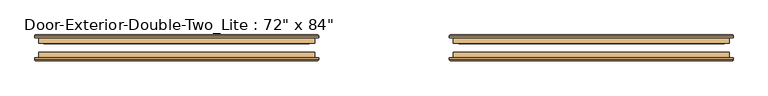
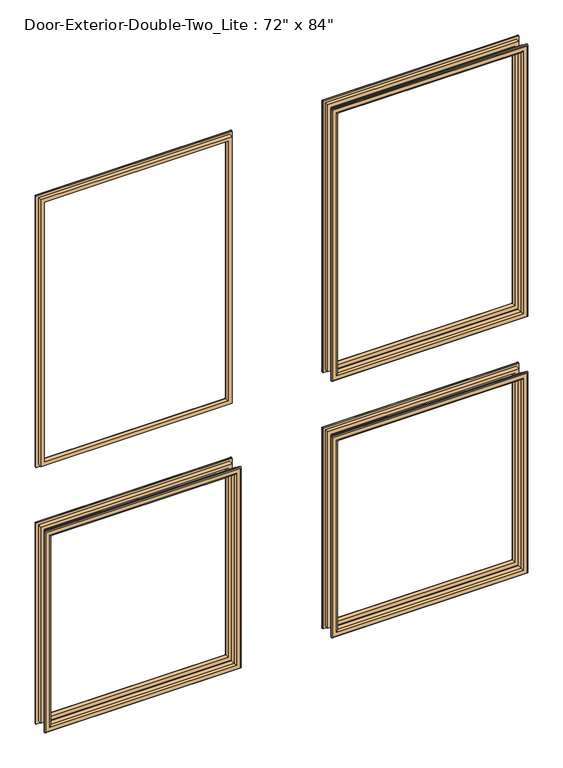
"""IFC4 building model written with IfcOpenShell, lengths in millimetres: door geometry."""

from ifc_helpers import new_model, si_unit, frame, origin, place, context, project, spatial, ellipse_curve, source, transform, mapped, element, save
from ifc_brep_helpers import plane_surface, cylinder_surface, advanced_brep


def door_549a8064(model_context):
    return source(origin(), model_context, "Body", "AdvancedBrep", [
        advanced_brep(
        [(-762.0, 69.85, 914.4), (-762.0, 82.55, 914.4), (-762.0, 82.55, 254.0), (-762.0, 69.85, 254.0), (-750.0, 83.55, 902.4), (-750.0, 69.85, 902.4), (-750.0, 69.85, 266.0), (-750.0, 83.55, 266.0), (-755.0, 88.55, 907.4), (-755.0, 88.55, 261.0), (-770.0, 86.55, 922.4), (-768.0, 88.55, 920.4), (-768.0, 88.55, 248.0), (-770.0, 86.55, 246.0), (-770.0, 82.55, 922.4), (-770.0, 82.55, 246.0), (-152.4, 82.55, 254.0), (-152.4, 69.85, 254.0), (-164.4, 69.85, 266.0), (-164.4, 83.55, 266.0), (-159.4, 88.55, 261.0), (-146.4, 88.55, 248.0), (-144.4, 86.55, 246.0), (-144.4, 82.55, 246.0), (-152.4, 82.55, 914.4), (-152.4, 69.85, 914.4), (-164.4, 69.85, 902.4), (-164.4, 83.55, 902.4), (-159.4, 88.55, 907.4), (-146.4, 88.55, 920.4), (-144.4, 86.55, 922.4), (-144.4, 82.55, 922.4)],
        [
            (0, 1),
            (1, 2),
            (2, 3),
            (3, 0),
            (4, 5),
            (5, 6),
            (6, 7),
            (7, 4),
            (8, 4, ellipse_curve(frame((-755.0, 83.55, 907.4), z_axis=(-0.7071067811865475, 0.0, -0.7071067811865475), x_axis=(-0.7071067811865474, 0.0, 0.7071067811865476)), 7.0710678, 5.0)),
            (7, 9, ellipse_curve(frame((-755.0, 83.55, 261.0), z_axis=(-0.7071067811865475, 0.0, 0.7071067811865475), x_axis=(0.7071067811865474, 0.0, 0.7071067811865476)), 7.0710678, 5.0)),
            (9, 8),
            (10, 11, ellipse_curve(frame((-768.0, 86.55, 920.4), z_axis=(-0.7071067811865475, 0.0, -0.7071067811865475), x_axis=(-0.7071067811865474, 0.0, 0.7071067811865476)), 2.8284271, 2.0)),
            (11, 12),
            (12, 13, ellipse_curve(frame((-768.0, 86.55, 248.0), z_axis=(-0.7071067811865475, 0.0, 0.7071067811865475), x_axis=(0.7071067811865474, 0.0, 0.7071067811865476)), 2.8284271, 2.0)),
            (13, 10),
            (14, 10),
            (13, 15),
            (15, 14),
            (2, 16),
            (16, 17),
            (17, 3),
            (6, 18),
            (18, 19),
            (19, 7),
            (19, 20, ellipse_curve(frame((-159.4, 83.55, 261.0), z_axis=(-0.7071067811865475, 0.0, -0.7071067811865475), x_axis=(-0.7071067811865476, 0.0, 0.7071067811865474)), 7.0710678, 5.0)),
            (20, 9),
            (12, 21),
            (21, 22, ellipse_curve(frame((-146.4, 86.55, 248.0), z_axis=(-0.7071067811865475, 0.0, -0.7071067811865475), x_axis=(-0.7071067811865476, 0.0, 0.7071067811865474)), 2.8284271, 2.0)),
            (22, 13),
            (22, 23),
            (23, 15),
            (16, 24),
            (24, 25),
            (25, 17),
            (18, 26),
            (26, 27),
            (27, 19),
            (27, 28, ellipse_curve(frame((-159.4, 83.55, 907.4), z_axis=(0.7071067811865475, 0.0, -0.7071067811865475), x_axis=(-0.7071067811865474, 0.0, -0.7071067811865476)), 7.0710678, 5.0)),
            (28, 20),
            (21, 29),
            (29, 30, ellipse_curve(frame((-146.4, 86.55, 920.4), z_axis=(0.7071067811865475, 0.0, -0.7071067811865475), x_axis=(-0.7071067811865474, 0.0, -0.7071067811865476)), 2.8284271, 2.0)),
            (30, 22),
            (30, 31),
            (31, 23),
            (31, 14),
            (1, 24),
            (0, 25),
            (5, 26),
            (4, 27),
            (8, 28),
            (11, 29),
            (10, 30),
        ],
        [
            plane_surface(frame((-762.0, 82.55, 914.4), z_axis=(-1.0, 0.0, 0.0), x_axis=(0.0, 0.0, -1.0))),
            plane_surface(frame((-750.0, 69.85, 902.4), z_axis=(1.0, 0.0, 0.0), x_axis=(0.0, 0.0, -1.0))),
            cylinder_surface(frame((-755.0, 83.55, 914.4), z_axis=(0.0, 0.0, 1.0), x_axis=(-1.0, 0.0, 0.0)), 5.0),
            cylinder_surface(frame((-768.0, 86.55, 914.4), z_axis=(0.0, 0.0, 1.0), x_axis=(-1.0, 0.0, 0.0)), 2.0),
            plane_surface(frame((-770.0, 86.55, 922.4), z_axis=(-1.0, 0.0, 0.0), x_axis=(0.0, 0.0, -1.0))),
            plane_surface(frame((-762.0, 82.55, 254.0), z_axis=(0.0, 0.0, -1.0), x_axis=(1.0, 0.0, 0.0))),
            plane_surface(frame((-750.0, 69.85, 266.0), z_axis=(0.0, 0.0, 1.0), x_axis=(1.0, 0.0, 0.0))),
            cylinder_surface(frame((-762.0, 83.55, 261.0), z_axis=(-1.0, 0.0, 0.0), x_axis=(0.0, 0.0, -1.0)), 5.0),
            cylinder_surface(frame((-762.0, 86.55, 248.0), z_axis=(-1.0, 0.0, 0.0), x_axis=(0.0, 0.0, -1.0)), 2.0),
            plane_surface(frame((-770.0, 86.55, 246.0), z_axis=(0.0, 0.0, -1.0), x_axis=(1.0, 0.0, 0.0))),
            plane_surface(frame((-152.4, 82.55, 254.0), z_axis=(1.0, 0.0, 0.0), x_axis=(0.0, 0.0, 1.0))),
            plane_surface(frame((-164.4, 69.85, 266.0), z_axis=(-1.0, 0.0, 0.0), x_axis=(0.0, 0.0, 1.0))),
            cylinder_surface(frame((-159.4, 83.55, 254.0), z_axis=(0.0, 0.0, -1.0), x_axis=(1.0, 0.0, 0.0)), 5.0),
            cylinder_surface(frame((-146.4, 86.55, 254.0), z_axis=(0.0, 0.0, -1.0), x_axis=(1.0, 0.0, 0.0)), 2.0),
            plane_surface(frame((-144.4, 86.55, 246.0), z_axis=(1.0, 0.0, 0.0), x_axis=(0.0, 0.0, 1.0))),
            plane_surface(frame((-144.4, 82.55, 922.4), z_axis=(0.0, -1.0, 0.0), x_axis=(-1.0, 0.0, 0.0))),
            plane_surface(frame((-152.4, 82.55, 914.4), z_axis=(0.0, 0.0, 1.0), x_axis=(-1.0, 0.0, 0.0))),
            plane_surface(frame((-152.4, 69.85, 914.4), z_axis=(0.0, -1.0, 0.0), x_axis=(-1.0, 0.0, 0.0))),
            plane_surface(frame((-164.4, 69.85, 902.4), z_axis=(0.0, 0.0, -1.0), x_axis=(-1.0, 0.0, 0.0))),
            cylinder_surface(frame((-152.4, 83.55, 907.4), z_axis=(1.0, 0.0, 0.0), x_axis=(0.0, 0.0, 1.0)), 5.0),
            plane_surface(frame((-159.4, 88.55, 907.4), z_axis=(0.0, 1.0, 0.0), x_axis=(-1.0, 0.0, 0.0))),
            cylinder_surface(frame((-152.4, 86.55, 920.4), z_axis=(1.0, 0.0, 0.0), x_axis=(0.0, 0.0, 1.0)), 2.0),
            plane_surface(frame((-144.4, 86.55, 922.4), z_axis=(0.0, 0.0, 1.0), x_axis=(-1.0, 0.0, 0.0))),
        ],
        [
            (0, [[1, 2, 3, 4]]),
            (1, [[5, 6, 7, 8]]),
            (2, [[9, -8, 10, 11]]),
            (3, [[12, 13, 14, 15]]),
            (4, [[16, -15, 17, 18]]),
            (5, [[-3, 19, 20, 21]]),
            (6, [[-7, 22, 23, 24]]),
            (7, [[-10, -24, 25, 26]]),
            (8, [[-14, 27, 28, 29]]),
            (9, [[-17, -29, 30, 31]]),
            (10, [[-20, 32, 33, 34]]),
            (11, [[-23, 35, 36, 37]]),
            (12, [[-25, -37, 38, 39]]),
            (13, [[-28, 40, 41, 42]]),
            (14, [[-30, -42, 43, 44]]),
            (15, [[-31, -44, 45, -18], [46, -32, -19, -2]]),
            (16, [[-33, -46, -1, 47]]),
            (17, [[-21, -34, -47, -4], [48, -35, -22, -6]]),
            (18, [[-36, -48, -5, 49]]),
            (19, [[-38, -49, -9, 50]]),
            (20, [[51, -40, -27, -13], [-26, -39, -50, -11]]),
            (21, [[-41, -51, -12, 52]]),
            (22, [[-43, -52, -16, -45]]),
        ],
    ),
        advanced_brep(
        [(152.4, 69.85, 914.4), (152.4, 82.55, 914.4), (152.4, 82.55, 254.0), (152.4, 69.85, 254.0), (164.4, 83.55, 902.4), (164.4, 69.85, 902.4), (164.4, 69.85, 266.0), (164.4, 83.55, 266.0), (159.4, 88.55, 907.4), (159.4, 88.55, 261.0), (144.4, 86.55, 922.4), (146.4, 88.55, 920.4), (146.4, 88.55, 248.0), (144.4, 86.55, 246.0), (144.4, 82.55, 922.4), (144.4, 82.55, 246.0), (762.0, 82.55, 254.0), (762.0, 69.85, 254.0), (750.0, 69.85, 266.0), (750.0, 83.55, 266.0), (755.0, 88.55, 261.0), (768.0, 88.55, 248.0), (770.0, 86.55, 246.0), (770.0, 82.55, 246.0), (762.0, 82.55, 914.4), (762.0, 69.85, 914.4), (750.0, 69.85, 902.4), (750.0, 83.55, 902.4), (755.0, 88.55, 907.4), (768.0, 88.55, 920.4), (770.0, 86.55, 922.4), (770.0, 82.55, 922.4)],
        [
            (0, 1),
            (1, 2),
            (2, 3),
            (3, 0),
            (4, 5),
            (5, 6),
            (6, 7),
            (7, 4),
            (8, 4, ellipse_curve(frame((159.4, 83.55, 907.4), z_axis=(-0.7071067811865475, 0.0, -0.7071067811865475), x_axis=(-0.7071067811865474, 0.0, 0.7071067811865476)), 7.0710678, 5.0)),
            (7, 9, ellipse_curve(frame((159.4, 83.55, 261.0), z_axis=(-0.7071067811865475, 0.0, 0.7071067811865475), x_axis=(0.7071067811865474, 0.0, 0.7071067811865476)), 7.0710678, 5.0)),
            (9, 8),
            (10, 11, ellipse_curve(frame((146.4, 86.55, 920.4), z_axis=(-0.7071067811865475, 0.0, -0.7071067811865475), x_axis=(-0.7071067811865474, 0.0, 0.7071067811865476)), 2.8284271, 2.0)),
            (11, 12),
            (12, 13, ellipse_curve(frame((146.4, 86.55, 248.0), z_axis=(-0.7071067811865475, 0.0, 0.7071067811865475), x_axis=(0.7071067811865474, 0.0, 0.7071067811865476)), 2.8284271, 2.0)),
            (13, 10),
            (14, 10),
            (13, 15),
            (15, 14),
            (2, 16),
            (16, 17),
            (17, 3),
            (6, 18),
            (18, 19),
            (19, 7),
            (19, 20, ellipse_curve(frame((755.0, 83.55, 261.0), z_axis=(-0.7071067811865475, 0.0, -0.7071067811865475), x_axis=(-0.7071067811865476, 0.0, 0.7071067811865474)), 7.0710678, 5.0)),
            (20, 9),
            (12, 21),
            (21, 22, ellipse_curve(frame((768.0, 86.55, 248.0), z_axis=(-0.7071067811865475, 0.0, -0.7071067811865475), x_axis=(-0.7071067811865476, 0.0, 0.7071067811865474)), 2.8284271, 2.0)),
            (22, 13),
            (22, 23),
            (23, 15),
            (16, 24),
            (24, 25),
            (25, 17),
            (18, 26),
            (26, 27),
            (27, 19),
            (27, 28, ellipse_curve(frame((755.0, 83.55, 907.4), z_axis=(0.7071067811865475, 0.0, -0.7071067811865475), x_axis=(-0.7071067811865474, 0.0, -0.7071067811865476)), 7.0710678, 5.0)),
            (28, 20),
            (21, 29),
            (29, 30, ellipse_curve(frame((768.0, 86.55, 920.4), z_axis=(0.7071067811865475, 0.0, -0.7071067811865475), x_axis=(-0.7071067811865474, 0.0, -0.7071067811865476)), 2.8284271, 2.0)),
            (30, 22),
            (30, 31),
            (31, 23),
            (31, 14),
            (1, 24),
            (0, 25),
            (5, 26),
            (4, 27),
            (8, 28),
            (11, 29),
            (10, 30),
        ],
        [
            plane_surface(frame((152.4, 82.55, 914.4), z_axis=(-1.0, 0.0, 0.0), x_axis=(0.0, 0.0, -1.0))),
            plane_surface(frame((164.4, 69.85, 902.4), z_axis=(1.0, 0.0, 0.0), x_axis=(0.0, 0.0, -1.0))),
            cylinder_surface(frame((159.4, 83.55, 914.4), z_axis=(0.0, 0.0, 1.0), x_axis=(-1.0, 0.0, 0.0)), 5.0),
            cylinder_surface(frame((146.4, 86.55, 914.4), z_axis=(0.0, 0.0, 1.0), x_axis=(-1.0, 0.0, 0.0)), 2.0),
            plane_surface(frame((144.4, 86.55, 922.4), z_axis=(-1.0, 0.0, 0.0), x_axis=(0.0, 0.0, -1.0))),
            plane_surface(frame((152.4, 82.55, 254.0), z_axis=(0.0, 0.0, -1.0), x_axis=(1.0, 0.0, 0.0))),
            plane_surface(frame((164.4, 69.85, 266.0), z_axis=(0.0, 0.0, 1.0), x_axis=(1.0, 0.0, 0.0))),
            cylinder_surface(frame((152.4, 83.55, 261.0), z_axis=(-1.0, 0.0, 0.0), x_axis=(0.0, 0.0, -1.0)), 5.0),
            cylinder_surface(frame((152.4, 86.55, 248.0), z_axis=(-1.0, 0.0, 0.0), x_axis=(0.0, 0.0, -1.0)), 2.0),
            plane_surface(frame((144.4, 86.55, 246.0), z_axis=(0.0, 0.0, -1.0), x_axis=(1.0, 0.0, 0.0))),
            plane_surface(frame((762.0, 82.55, 254.0), z_axis=(1.0, 0.0, 0.0), x_axis=(0.0, 0.0, 1.0))),
            plane_surface(frame((750.0, 69.85, 266.0), z_axis=(-1.0, 0.0, 0.0), x_axis=(0.0, 0.0, 1.0))),
            cylinder_surface(frame((755.0, 83.55, 254.0), z_axis=(0.0, 0.0, -1.0), x_axis=(1.0, 0.0, 0.0)), 5.0),
            cylinder_surface(frame((768.0, 86.55, 254.0), z_axis=(0.0, 0.0, -1.0), x_axis=(1.0, 0.0, 0.0)), 2.0),
            plane_surface(frame((770.0, 86.55, 246.0), z_axis=(1.0, 0.0, 0.0), x_axis=(0.0, 0.0, 1.0))),
            plane_surface(frame((770.0, 82.55, 922.4), z_axis=(0.0, -1.0, 0.0), x_axis=(-1.0, 0.0, 0.0))),
            plane_surface(frame((762.0, 82.55, 914.4), z_axis=(0.0, 0.0, 1.0), x_axis=(-1.0, 0.0, 0.0))),
            plane_surface(frame((762.0, 69.85, 914.4), z_axis=(0.0, -1.0, 0.0), x_axis=(-1.0, 0.0, 0.0))),
            plane_surface(frame((750.0, 69.85, 902.4), z_axis=(0.0, 0.0, -1.0), x_axis=(-1.0, 0.0, 0.0))),
            cylinder_surface(frame((762.0, 83.55, 907.4), z_axis=(1.0, 0.0, 0.0), x_axis=(0.0, 0.0, 1.0)), 5.0),
            plane_surface(frame((755.0, 88.55, 907.4), z_axis=(0.0, 1.0, 0.0), x_axis=(-1.0, 0.0, 0.0))),
            cylinder_surface(frame((762.0, 86.55, 920.4), z_axis=(1.0, 0.0, 0.0), x_axis=(0.0, 0.0, 1.0)), 2.0),
            plane_surface(frame((770.0, 86.55, 922.4), z_axis=(0.0, 0.0, 1.0), x_axis=(-1.0, 0.0, 0.0))),
        ],
        [
            (0, [[1, 2, 3, 4]]),
            (1, [[5, 6, 7, 8]]),
            (2, [[9, -8, 10, 11]]),
            (3, [[12, 13, 14, 15]]),
            (4, [[16, -15, 17, 18]]),
            (5, [[-3, 19, 20, 21]]),
            (6, [[-7, 22, 23, 24]]),
            (7, [[-10, -24, 25, 26]]),
            (8, [[-14, 27, 28, 29]]),
            (9, [[-17, -29, 30, 31]]),
            (10, [[-20, 32, 33, 34]]),
            (11, [[-23, 35, 36, 37]]),
            (12, [[-25, -37, 38, 39]]),
            (13, [[-28, 40, 41, 42]]),
            (14, [[-30, -42, 43, 44]]),
            (15, [[-31, -44, 45, -18], [46, -32, -19, -2]]),
            (16, [[-33, -46, -1, 47]]),
            (17, [[-21, -34, -47, -4], [48, -35, -22, -6]]),
            (18, [[-36, -48, -5, 49]]),
            (19, [[-38, -49, -9, 50]]),
            (20, [[51, -40, -27, -13], [-26, -39, -50, -11]]),
            (21, [[-41, -51, -12, 52]]),
            (22, [[-43, -52, -16, -45]]),
        ],
    ),
        advanced_brep(
        [(152.4, 69.85, 2016.125), (152.4, 82.55, 2016.125), (152.4, 82.55, 1117.6), (152.4, 69.85, 1117.6), (164.4, 83.55, 2004.125), (164.4, 69.85, 2004.125), (164.4, 69.85, 1129.6), (164.4, 83.55, 1129.6), (159.4, 88.55, 2009.125), (159.4, 88.55, 1124.6), (144.4, 86.55, 2024.125), (146.4, 88.55, 2022.125), (146.4, 88.55, 1111.6), (144.4, 86.55, 1109.6), (144.4, 82.55, 2024.125), (144.4, 82.55, 1109.6), (762.0, 82.55, 1117.6), (762.0, 69.85, 1117.6), (750.0, 69.85, 1129.6), (750.0, 83.55, 1129.6), (755.0, 88.55, 1124.6), (768.0, 88.55, 1111.6), (770.0, 86.55, 1109.6), (770.0, 82.55, 1109.6), (762.0, 82.55, 2016.125), (762.0, 69.85, 2016.125), (750.0, 69.85, 2004.125), (750.0, 83.55, 2004.125), (755.0, 88.55, 2009.125), (768.0, 88.55, 2022.125), (770.0, 86.55, 2024.125), (770.0, 82.55, 2024.125)],
        [
            (0, 1),
            (1, 2),
            (2, 3),
            (3, 0),
            (4, 5),
            (5, 6),
            (6, 7),
            (7, 4),
            (8, 4, ellipse_curve(frame((159.4, 83.55, 2009.125), z_axis=(-0.7071067811865475, 0.0, -0.7071067811865475), x_axis=(-0.7071067811865474, 0.0, 0.7071067811865476)), 7.0710678, 5.0)),
            (7, 9, ellipse_curve(frame((159.4, 83.55, 1124.6), z_axis=(-0.7071067811865475, 0.0, 0.7071067811865475), x_axis=(0.7071067811865474, 0.0, 0.7071067811865476)), 7.0710678, 5.0)),
            (9, 8),
            (10, 11, ellipse_curve(frame((146.4, 86.55, 2022.125), z_axis=(-0.7071067811865475, 0.0, -0.7071067811865475), x_axis=(-0.7071067811865474, 0.0, 0.7071067811865476)), 2.8284271, 2.0)),
            (11, 12),
            (12, 13, ellipse_curve(frame((146.4, 86.55, 1111.6), z_axis=(-0.7071067811865475, 0.0, 0.7071067811865475), x_axis=(0.7071067811865474, 0.0, 0.7071067811865476)), 2.8284271, 2.0)),
            (13, 10),
            (14, 10),
            (13, 15),
            (15, 14),
            (2, 16),
            (16, 17),
            (17, 3),
            (6, 18),
            (18, 19),
            (19, 7),
            (19, 20, ellipse_curve(frame((755.0, 83.55, 1124.6), z_axis=(-0.7071067811865475, 0.0, -0.7071067811865475), x_axis=(-0.7071067811865476, 0.0, 0.7071067811865474)), 7.0710678, 5.0)),
            (20, 9),
            (12, 21),
            (21, 22, ellipse_curve(frame((768.0, 86.55, 1111.6), z_axis=(-0.7071067811865475, 0.0, -0.7071067811865475), x_axis=(-0.7071067811865476, 0.0, 0.7071067811865474)), 2.8284271, 2.0)),
            (22, 13),
            (22, 23),
            (23, 15),
            (16, 24),
            (24, 25),
            (25, 17),
            (18, 26),
            (26, 27),
            (27, 19),
            (27, 28, ellipse_curve(frame((755.0, 83.55, 2009.125), z_axis=(0.7071067811865475, 0.0, -0.7071067811865475), x_axis=(-0.7071067811865474, 0.0, -0.7071067811865476)), 7.0710678, 5.0)),
            (28, 20),
            (21, 29),
            (29, 30, ellipse_curve(frame((768.0, 86.55, 2022.125), z_axis=(0.7071067811865475, 0.0, -0.7071067811865475), x_axis=(-0.7071067811865474, 0.0, -0.7071067811865476)), 2.8284271, 2.0)),
            (30, 22),
            (30, 31),
            (31, 23),
            (31, 14),
            (1, 24),
            (0, 25),
            (5, 26),
            (4, 27),
            (8, 28),
            (11, 29),
            (10, 30),
        ],
        [
            plane_surface(frame((152.4, 82.55, 2016.125), z_axis=(-1.0, 0.0, 0.0), x_axis=(0.0, 0.0, -1.0))),
            plane_surface(frame((164.4, 69.85, 2004.125), z_axis=(1.0, 0.0, 0.0), x_axis=(0.0, 0.0, -1.0))),
            cylinder_surface(frame((159.4, 83.55, 2016.125), z_axis=(0.0, 0.0, 1.0), x_axis=(-1.0, 0.0, 0.0)), 5.0),
            cylinder_surface(frame((146.4, 86.55, 2016.125), z_axis=(0.0, 0.0, 1.0), x_axis=(-1.0, 0.0, 0.0)), 2.0),
            plane_surface(frame((144.4, 86.55, 2024.125), z_axis=(-1.0, 0.0, 0.0), x_axis=(0.0, 0.0, -1.0))),
            plane_surface(frame((152.4, 82.55, 1117.6), z_axis=(0.0, 0.0, -1.0), x_axis=(1.0, 0.0, 0.0))),
            plane_surface(frame((164.4, 69.85, 1129.6), z_axis=(0.0, 0.0, 1.0), x_axis=(1.0, 0.0, 0.0))),
            cylinder_surface(frame((152.4, 83.55, 1124.6), z_axis=(-1.0, 0.0, 0.0), x_axis=(0.0, 0.0, -1.0)), 5.0),
            cylinder_surface(frame((152.4, 86.55, 1111.6), z_axis=(-1.0, 0.0, 0.0), x_axis=(0.0, 0.0, -1.0)), 2.0),
            plane_surface(frame((144.4, 86.55, 1109.6), z_axis=(0.0, 0.0, -1.0), x_axis=(1.0, 0.0, 0.0))),
            plane_surface(frame((762.0, 82.55, 1117.6), z_axis=(1.0, 0.0, 0.0), x_axis=(0.0, 0.0, 1.0))),
            plane_surface(frame((750.0, 69.85, 1129.6), z_axis=(-1.0, 0.0, 0.0), x_axis=(0.0, 0.0, 1.0))),
            cylinder_surface(frame((755.0, 83.55, 1117.6), z_axis=(0.0, 0.0, -1.0), x_axis=(1.0, 0.0, 0.0)), 5.0),
            cylinder_surface(frame((768.0, 86.55, 1117.6), z_axis=(0.0, 0.0, -1.0), x_axis=(1.0, 0.0, 0.0)), 2.0),
            plane_surface(frame((770.0, 86.55, 1109.6), z_axis=(1.0, 0.0, 0.0), x_axis=(0.0, 0.0, 1.0))),
            plane_surface(frame((770.0, 82.55, 2024.125), z_axis=(0.0, -1.0, 0.0), x_axis=(-1.0, 0.0, 0.0))),
            plane_surface(frame((762.0, 82.55, 2016.125), z_axis=(0.0, 0.0, 1.0), x_axis=(-1.0, 0.0, 0.0))),
            plane_surface(frame((762.0, 69.85, 2016.125), z_axis=(0.0, -1.0, 0.0), x_axis=(-1.0, 0.0, 0.0))),
            plane_surface(frame((750.0, 69.85, 2004.125), z_axis=(0.0, 0.0, -1.0), x_axis=(-1.0, 0.0, 0.0))),
            cylinder_surface(frame((762.0, 83.55, 2009.125), z_axis=(1.0, 0.0, 0.0), x_axis=(0.0, 0.0, 1.0)), 5.0),
            plane_surface(frame((755.0, 88.55, 2009.125), z_axis=(0.0, 1.0, 0.0), x_axis=(-1.0, 0.0, 0.0))),
            cylinder_surface(frame((762.0, 86.55, 2022.125), z_axis=(1.0, 0.0, 0.0), x_axis=(0.0, 0.0, 1.0)), 2.0),
            plane_surface(frame((770.0, 86.55, 2024.125), z_axis=(0.0, 0.0, 1.0), x_axis=(-1.0, 0.0, 0.0))),
        ],
        [
            (0, [[1, 2, 3, 4]]),
            (1, [[5, 6, 7, 8]]),
            (2, [[9, -8, 10, 11]]),
            (3, [[12, 13, 14, 15]]),
            (4, [[16, -15, 17, 18]]),
            (5, [[-3, 19, 20, 21]]),
            (6, [[-7, 22, 23, 24]]),
            (7, [[-10, -24, 25, 26]]),
            (8, [[-14, 27, 28, 29]]),
            (9, [[-17, -29, 30, 31]]),
            (10, [[-20, 32, 33, 34]]),
            (11, [[-23, 35, 36, 37]]),
            (12, [[-25, -37, 38, 39]]),
            (13, [[-28, 40, 41, 42]]),
            (14, [[-30, -42, 43, 44]]),
            (15, [[-31, -44, 45, -18], [46, -32, -19, -2]]),
            (16, [[-33, -46, -1, 47]]),
            (17, [[-21, -34, -47, -4], [48, -35, -22, -6]]),
            (18, [[-36, -48, -5, 49]]),
            (19, [[-38, -49, -9, 50]]),
            (20, [[51, -40, -27, -13], [-26, -39, -50, -11]]),
            (21, [[-41, -51, -12, 52]]),
            (22, [[-43, -52, -16, -45]]),
        ],
    ),
        advanced_brep(
        [(-762.0, 69.85, 2016.125), (-762.0, 82.55, 2016.125), (-762.0, 82.55, 1117.6), (-762.0, 69.85, 1117.6), (-750.0, 83.55, 2004.125), (-750.0, 69.85, 2004.125), (-750.0, 69.85, 1129.6), (-750.0, 83.55, 1129.6), (-755.0, 88.55, 2009.125), (-755.0, 88.55, 1124.6), (-770.0, 86.55, 2024.125), (-768.0, 88.55, 2022.125), (-768.0, 88.55, 1111.6), (-770.0, 86.55, 1109.6), (-770.0, 82.55, 2024.125), (-770.0, 82.55, 1109.6), (-152.4, 82.55, 1117.6), (-152.4, 69.85, 1117.6), (-164.4, 69.85, 1129.6), (-164.4, 83.55, 1129.6), (-159.4, 88.55, 1124.6), (-146.4, 88.55, 1111.6), (-144.4, 86.55, 1109.6), (-144.4, 82.55, 1109.6), (-152.4, 82.55, 2016.125), (-152.4, 69.85, 2016.125), (-164.4, 69.85, 2004.125), (-164.4, 83.55, 2004.125), (-159.4, 88.55, 2009.125), (-146.4, 88.55, 2022.125), (-144.4, 86.55, 2024.125), (-144.4, 82.55, 2024.125)],
        [
            (0, 1),
            (1, 2),
            (2, 3),
            (3, 0),
            (4, 5),
            (5, 6),
            (6, 7),
            (7, 4),
            (8, 4, ellipse_curve(frame((-755.0, 83.55, 2009.125), z_axis=(-0.7071067811865475, 0.0, -0.7071067811865475), x_axis=(-0.7071067811865474, 0.0, 0.7071067811865476)), 7.0710678, 5.0)),
            (7, 9, ellipse_curve(frame((-755.0, 83.55, 1124.6), z_axis=(-0.7071067811865475, 0.0, 0.7071067811865475), x_axis=(0.7071067811865474, 0.0, 0.7071067811865476)), 7.0710678, 5.0)),
            (9, 8),
            (10, 11, ellipse_curve(frame((-768.0, 86.55, 2022.125), z_axis=(-0.7071067811865475, 0.0, -0.7071067811865475), x_axis=(-0.7071067811865474, 0.0, 0.7071067811865476)), 2.8284271, 2.0)),
            (11, 12),
            (12, 13, ellipse_curve(frame((-768.0, 86.55, 1111.6), z_axis=(-0.7071067811865475, 0.0, 0.7071067811865475), x_axis=(0.7071067811865474, 0.0, 0.7071067811865476)), 2.8284271, 2.0)),
            (13, 10),
            (14, 10),
            (13, 15),
            (15, 14),
            (2, 16),
            (16, 17),
            (17, 3),
            (6, 18),
            (18, 19),
            (19, 7),
            (19, 20, ellipse_curve(frame((-159.4, 83.55, 1124.6), z_axis=(-0.7071067811865475, 0.0, -0.7071067811865475), x_axis=(-0.7071067811865476, 0.0, 0.7071067811865474)), 7.0710678, 5.0)),
            (20, 9),
            (12, 21),
            (21, 22, ellipse_curve(frame((-146.4, 86.55, 1111.6), z_axis=(-0.7071067811865475, 0.0, -0.7071067811865475), x_axis=(-0.7071067811865476, 0.0, 0.7071067811865474)), 2.8284271, 2.0)),
            (22, 13),
            (22, 23),
            (23, 15),
            (16, 24),
            (24, 25),
            (25, 17),
            (18, 26),
            (26, 27),
            (27, 19),
            (27, 28, ellipse_curve(frame((-159.4, 83.55, 2009.125), z_axis=(0.7071067811865475, 0.0, -0.7071067811865475), x_axis=(-0.7071067811865474, 0.0, -0.7071067811865476)), 7.0710678, 5.0)),
            (28, 20),
            (21, 29),
            (29, 30, ellipse_curve(frame((-146.4, 86.55, 2022.125), z_axis=(0.7071067811865475, 0.0, -0.7071067811865475), x_axis=(-0.7071067811865474, 0.0, -0.7071067811865476)), 2.8284271, 2.0)),
            (30, 22),
            (30, 31),
            (31, 23),
            (31, 14),
            (1, 24),
            (0, 25),
            (5, 26),
            (4, 27),
            (8, 28),
            (11, 29),
            (10, 30),
        ],
        [
            plane_surface(frame((-762.0, 82.55, 2016.125), z_axis=(-1.0, 0.0, 0.0), x_axis=(0.0, 0.0, -1.0))),
            plane_surface(frame((-750.0, 69.85, 2004.125), z_axis=(1.0, 0.0, 0.0), x_axis=(0.0, 0.0, -1.0))),
            cylinder_surface(frame((-755.0, 83.55, 2016.125), z_axis=(0.0, 0.0, 1.0), x_axis=(-1.0, 0.0, 0.0)), 5.0),
            cylinder_surface(frame((-768.0, 86.55, 2016.125), z_axis=(0.0, 0.0, 1.0), x_axis=(-1.0, 0.0, 0.0)), 2.0),
            plane_surface(frame((-770.0, 86.55, 2024.125), z_axis=(-1.0, 0.0, 0.0), x_axis=(0.0, 0.0, -1.0))),
            plane_surface(frame((-762.0, 82.55, 1117.6), z_axis=(0.0, 0.0, -1.0), x_axis=(1.0, 0.0, 0.0))),
            plane_surface(frame((-750.0, 69.85, 1129.6), z_axis=(0.0, 0.0, 1.0), x_axis=(1.0, 0.0, 0.0))),
            cylinder_surface(frame((-762.0, 83.55, 1124.6), z_axis=(-1.0, 0.0, 0.0), x_axis=(0.0, 0.0, -1.0)), 5.0),
            cylinder_surface(frame((-762.0, 86.55, 1111.6), z_axis=(-1.0, 0.0, 0.0), x_axis=(0.0, 0.0, -1.0)), 2.0),
            plane_surface(frame((-770.0, 86.55, 1109.6), z_axis=(0.0, 0.0, -1.0), x_axis=(1.0, 0.0, 0.0))),
            plane_surface(frame((-152.4, 82.55, 1117.6), z_axis=(1.0, 0.0, 0.0), x_axis=(0.0, 0.0, 1.0))),
            plane_surface(frame((-164.4, 69.85, 1129.6), z_axis=(-1.0, 0.0, 0.0), x_axis=(0.0, 0.0, 1.0))),
            cylinder_surface(frame((-159.4, 83.55, 1117.6), z_axis=(0.0, 0.0, -1.0), x_axis=(1.0, 0.0, 0.0)), 5.0),
            cylinder_surface(frame((-146.4, 86.55, 1117.6), z_axis=(0.0, 0.0, -1.0), x_axis=(1.0, 0.0, 0.0)), 2.0),
            plane_surface(frame((-144.4, 86.55, 1109.6), z_axis=(1.0, 0.0, 0.0), x_axis=(0.0, 0.0, 1.0))),
            plane_surface(frame((-144.4, 82.55, 2024.125), z_axis=(0.0, -1.0, 0.0), x_axis=(-1.0, 0.0, 0.0))),
            plane_surface(frame((-152.4, 82.55, 2016.125), z_axis=(0.0, 0.0, 1.0), x_axis=(-1.0, 0.0, 0.0))),
            plane_surface(frame((-152.4, 69.85, 2016.125), z_axis=(0.0, -1.0, 0.0), x_axis=(-1.0, 0.0, 0.0))),
            plane_surface(frame((-164.4, 69.85, 2004.125), z_axis=(0.0, 0.0, -1.0), x_axis=(-1.0, 0.0, 0.0))),
            cylinder_surface(frame((-152.4, 83.55, 2009.125), z_axis=(1.0, 0.0, 0.0), x_axis=(0.0, 0.0, 1.0)), 5.0),
            plane_surface(frame((-159.4, 88.55, 2009.125), z_axis=(0.0, 1.0, 0.0), x_axis=(-1.0, 0.0, 0.0))),
            cylinder_surface(frame((-152.4, 86.55, 2022.125), z_axis=(1.0, 0.0, 0.0), x_axis=(0.0, 0.0, 1.0)), 2.0),
            plane_surface(frame((-144.4, 86.55, 2024.125), z_axis=(0.0, 0.0, 1.0), x_axis=(-1.0, 0.0, 0.0))),
        ],
        [
            (0, [[1, 2, 3, 4]]),
            (1, [[5, 6, 7, 8]]),
            (2, [[9, -8, 10, 11]]),
            (3, [[12, 13, 14, 15]]),
            (4, [[16, -15, 17, 18]]),
            (5, [[-3, 19, 20, 21]]),
            (6, [[-7, 22, 23, 24]]),
            (7, [[-10, -24, 25, 26]]),
            (8, [[-14, 27, 28, 29]]),
            (9, [[-17, -29, 30, 31]]),
            (10, [[-20, 32, 33, 34]]),
            (11, [[-23, 35, 36, 37]]),
            (12, [[-25, -37, 38, 39]]),
            (13, [[-28, 40, 41, 42]]),
            (14, [[-30, -42, 43, 44]]),
            (15, [[-31, -44, 45, -18], [46, -32, -19, -2]]),
            (16, [[-33, -46, -1, 47]]),
            (17, [[-21, -34, -47, -4], [48, -35, -22, -6]]),
            (18, [[-36, -48, -5, 49]]),
            (19, [[-38, -49, -9, 50]]),
            (20, [[51, -40, -27, -13], [-26, -39, -50, -11]]),
            (21, [[-41, -51, -12, 52]]),
            (22, [[-43, -52, -16, -45]]),
        ],
    ),
        advanced_brep(
        [(-762.0, 50.8, 254.0), (-762.0, 38.1, 254.0), (-762.0, 38.1, 914.4), (-762.0, 50.8, 914.4), (-750.0, 37.1, 266.0), (-750.0, 50.8, 266.0), (-750.0, 50.8, 902.4), (-750.0, 37.1, 902.4), (-755.0, 32.1, 261.0), (-755.0, 32.1, 907.4), (-770.0, 34.1, 246.0), (-768.0, 32.1, 248.0), (-768.0, 32.1, 920.4), (-770.0, 34.1, 922.4), (-770.0, 38.1, 246.0), (-770.0, 38.1, 922.4), (-152.4, 38.1, 914.4), (-152.4, 50.8, 914.4), (-164.4, 50.8, 902.4), (-164.4, 37.1, 902.4), (-159.4, 32.1, 907.4), (-146.4, 32.1, 920.4), (-144.4, 34.1, 922.4), (-144.4, 38.1, 922.4), (-152.4, 38.1, 254.0), (-152.4, 50.8, 254.0), (-164.4, 50.8, 266.0), (-164.4, 37.1, 266.0), (-159.4, 32.1, 261.0), (-146.4, 32.1, 248.0), (-144.4, 34.1, 246.0), (-144.4, 38.1, 246.0)],
        [
            (0, 1),
            (1, 2),
            (2, 3),
            (3, 0),
            (4, 5),
            (5, 6),
            (6, 7),
            (7, 4),
            (8, 4, ellipse_curve(frame((-755.0, 37.1, 261.0), z_axis=(-0.7071067811865475, 0.0, 0.7071067811865475), x_axis=(-0.7071067811865474, 0.0, -0.7071067811865476)), 7.0710678, 5.0)),
            (7, 9, ellipse_curve(frame((-755.0, 37.1, 907.4), z_axis=(-0.7071067811865475, 0.0, -0.7071067811865475), x_axis=(0.7071067811865474, 0.0, -0.7071067811865476)), 7.0710678, 5.0)),
            (9, 8),
            (10, 11, ellipse_curve(frame((-768.0, 34.1, 248.0), z_axis=(-0.7071067811865475, 0.0, 0.7071067811865475), x_axis=(-0.7071067811865474, 0.0, -0.7071067811865476)), 2.8284271, 2.0)),
            (11, 12),
            (12, 13, ellipse_curve(frame((-768.0, 34.1, 920.4), z_axis=(-0.7071067811865475, 0.0, -0.7071067811865475), x_axis=(0.7071067811865474, 0.0, -0.7071067811865476)), 2.8284271, 2.0)),
            (13, 10),
            (14, 10),
            (13, 15),
            (15, 14),
            (2, 16),
            (16, 17),
            (17, 3),
            (6, 18),
            (18, 19),
            (19, 7),
            (19, 20, ellipse_curve(frame((-159.4, 37.1, 907.4), z_axis=(-0.7071067811865475, 0.0, 0.7071067811865475), x_axis=(-0.7071067811865476, 0.0, -0.7071067811865474)), 7.0710678, 5.0)),
            (20, 9),
            (12, 21),
            (21, 22, ellipse_curve(frame((-146.4, 34.1, 920.4), z_axis=(-0.7071067811865475, 0.0, 0.7071067811865475), x_axis=(-0.7071067811865476, 0.0, -0.7071067811865474)), 2.8284271, 2.0)),
            (22, 13),
            (22, 23),
            (23, 15),
            (16, 24),
            (24, 25),
            (25, 17),
            (18, 26),
            (26, 27),
            (27, 19),
            (27, 28, ellipse_curve(frame((-159.4, 37.1, 261.0), z_axis=(0.7071067811865475, 0.0, 0.7071067811865475), x_axis=(-0.7071067811865474, 0.0, 0.7071067811865476)), 7.0710678, 5.0)),
            (28, 20),
            (21, 29),
            (29, 30, ellipse_curve(frame((-146.4, 34.1, 248.0), z_axis=(0.7071067811865475, 0.0, 0.7071067811865475), x_axis=(-0.7071067811865474, 0.0, 0.7071067811865476)), 2.8284271, 2.0)),
            (30, 22),
            (30, 31),
            (31, 23),
            (31, 14),
            (1, 24),
            (0, 25),
            (5, 26),
            (4, 27),
            (8, 28),
            (11, 29),
            (10, 30),
        ],
        [
            plane_surface(frame((-762.0, 38.1, 254.0), z_axis=(-1.0, 0.0, 0.0), x_axis=(0.0, 0.0, 1.0))),
            plane_surface(frame((-750.0, 50.8, 266.0), z_axis=(1.0, 0.0, 0.0), x_axis=(0.0, 0.0, 1.0))),
            cylinder_surface(frame((-755.0, 37.1, 254.0), z_axis=(0.0, 0.0, -1.0), x_axis=(-1.0, 0.0, 0.0)), 5.0),
            cylinder_surface(frame((-768.0, 34.1, 254.0), z_axis=(0.0, 0.0, -1.0), x_axis=(-1.0, 0.0, 0.0)), 2.0),
            plane_surface(frame((-770.0, 34.1, 246.0), z_axis=(-1.0, 0.0, 0.0), x_axis=(0.0, 0.0, 1.0))),
            plane_surface(frame((-762.0, 38.1, 914.4), z_axis=(0.0, 0.0, 1.0), x_axis=(1.0, 0.0, 0.0))),
            plane_surface(frame((-750.0, 50.8, 902.4), z_axis=(0.0, 0.0, -1.0), x_axis=(1.0, 0.0, 0.0))),
            cylinder_surface(frame((-762.0, 37.1, 907.4), z_axis=(-1.0, 0.0, 0.0), x_axis=(0.0, 0.0, 1.0)), 5.0),
            cylinder_surface(frame((-762.0, 34.1, 920.4), z_axis=(-1.0, 0.0, 0.0), x_axis=(0.0, 0.0, 1.0)), 2.0),
            plane_surface(frame((-770.0, 34.1, 922.4), z_axis=(0.0, 0.0, 1.0), x_axis=(1.0, 0.0, 0.0))),
            plane_surface(frame((-152.4, 38.1, 914.4), z_axis=(1.0, 0.0, 0.0), x_axis=(0.0, 0.0, -1.0))),
            plane_surface(frame((-164.4, 50.8, 902.4), z_axis=(-1.0, 0.0, 0.0), x_axis=(0.0, 0.0, -1.0))),
            cylinder_surface(frame((-159.4, 37.1, 914.4), z_axis=(0.0, 0.0, 1.0), x_axis=(1.0, 0.0, 0.0)), 5.0),
            cylinder_surface(frame((-146.4, 34.1, 914.4), z_axis=(0.0, 0.0, 1.0), x_axis=(1.0, 0.0, 0.0)), 2.0),
            plane_surface(frame((-144.4, 34.1, 922.4), z_axis=(1.0, 0.0, 0.0), x_axis=(0.0, 0.0, -1.0))),
            plane_surface(frame((-144.4, 38.1, 246.0), z_axis=(0.0, 1.0, 0.0), x_axis=(-1.0, 0.0, 0.0))),
            plane_surface(frame((-152.4, 38.1, 254.0), z_axis=(0.0, 0.0, -1.0), x_axis=(-1.0, 0.0, 0.0))),
            plane_surface(frame((-152.4, 50.8, 254.0), z_axis=(0.0, 1.0, 0.0), x_axis=(-1.0, 0.0, 0.0))),
            plane_surface(frame((-164.4, 50.8, 266.0), z_axis=(0.0, 0.0, 1.0), x_axis=(-1.0, 0.0, 0.0))),
            cylinder_surface(frame((-152.4, 37.1, 261.0), z_axis=(1.0, 0.0, 0.0), x_axis=(0.0, 0.0, -1.0)), 5.0),
            plane_surface(frame((-159.4, 32.1, 261.0), z_axis=(0.0, -1.0, 0.0), x_axis=(-1.0, 0.0, 0.0))),
            cylinder_surface(frame((-152.4, 34.1, 248.0), z_axis=(1.0, 0.0, 0.0), x_axis=(0.0, 0.0, -1.0)), 2.0),
            plane_surface(frame((-144.4, 34.1, 246.0), z_axis=(0.0, 0.0, -1.0), x_axis=(-1.0, 0.0, 0.0))),
        ],
        [
            (0, [[1, 2, 3, 4]]),
            (1, [[5, 6, 7, 8]]),
            (2, [[9, -8, 10, 11]]),
            (3, [[12, 13, 14, 15]]),
            (4, [[16, -15, 17, 18]]),
            (5, [[-3, 19, 20, 21]]),
            (6, [[-7, 22, 23, 24]]),
            (7, [[-10, -24, 25, 26]]),
            (8, [[-14, 27, 28, 29]]),
            (9, [[-17, -29, 30, 31]]),
            (10, [[-20, 32, 33, 34]]),
            (11, [[-23, 35, 36, 37]]),
            (12, [[-25, -37, 38, 39]]),
            (13, [[-28, 40, 41, 42]]),
            (14, [[-30, -42, 43, 44]]),
            (15, [[-31, -44, 45, -18], [46, -32, -19, -2]]),
            (16, [[-33, -46, -1, 47]]),
            (17, [[-21, -34, -47, -4], [48, -35, -22, -6]]),
            (18, [[-36, -48, -5, 49]]),
            (19, [[-38, -49, -9, 50]]),
            (20, [[51, -40, -27, -13], [-26, -39, -50, -11]]),
            (21, [[-41, -51, -12, 52]]),
            (22, [[-43, -52, -16, -45]]),
        ],
    ),
        advanced_brep(
        [(152.4, 50.8, 254.0), (152.4, 38.1, 254.0), (152.4, 38.1, 914.4), (152.4, 50.8, 914.4), (164.4, 37.1, 266.0), (164.4, 50.8, 266.0), (164.4, 50.8, 902.4), (164.4, 37.1, 902.4), (159.4, 32.1, 261.0), (159.4, 32.1, 907.4), (144.4, 34.1, 246.0), (146.4, 32.1, 248.0), (146.4, 32.1, 920.4), (144.4, 34.1, 922.4), (144.4, 38.1, 246.0), (144.4, 38.1, 922.4), (762.0, 38.1, 914.4), (762.0, 50.8, 914.4), (750.0, 50.8, 902.4), (750.0, 37.1, 902.4), (755.0, 32.1, 907.4), (768.0, 32.1, 920.4), (770.0, 34.1, 922.4), (770.0, 38.1, 922.4), (762.0, 38.1, 254.0), (762.0, 50.8, 254.0), (750.0, 50.8, 266.0), (750.0, 37.1, 266.0), (755.0, 32.1, 261.0), (768.0, 32.1, 248.0), (770.0, 34.1, 246.0), (770.0, 38.1, 246.0)],
        [
            (0, 1),
            (1, 2),
            (2, 3),
            (3, 0),
            (4, 5),
            (5, 6),
            (6, 7),
            (7, 4),
            (8, 4, ellipse_curve(frame((159.4, 37.1, 261.0), z_axis=(-0.7071067811865475, 0.0, 0.7071067811865475), x_axis=(-0.7071067811865474, 0.0, -0.7071067811865476)), 7.0710678, 5.0)),
            (7, 9, ellipse_curve(frame((159.4, 37.1, 907.4), z_axis=(-0.7071067811865475, 0.0, -0.7071067811865475), x_axis=(0.7071067811865474, 0.0, -0.7071067811865476)), 7.0710678, 5.0)),
            (9, 8),
            (10, 11, ellipse_curve(frame((146.4, 34.1, 248.0), z_axis=(-0.7071067811865475, 0.0, 0.7071067811865475), x_axis=(-0.7071067811865474, 0.0, -0.7071067811865476)), 2.8284271, 2.0)),
            (11, 12),
            (12, 13, ellipse_curve(frame((146.4, 34.1, 920.4), z_axis=(-0.7071067811865475, 0.0, -0.7071067811865475), x_axis=(0.7071067811865474, 0.0, -0.7071067811865476)), 2.8284271, 2.0)),
            (13, 10),
            (14, 10),
            (13, 15),
            (15, 14),
            (2, 16),
            (16, 17),
            (17, 3),
            (6, 18),
            (18, 19),
            (19, 7),
            (19, 20, ellipse_curve(frame((755.0, 37.1, 907.4), z_axis=(-0.7071067811865475, 0.0, 0.7071067811865475), x_axis=(-0.7071067811865476, 0.0, -0.7071067811865474)), 7.0710678, 5.0)),
            (20, 9),
            (12, 21),
            (21, 22, ellipse_curve(frame((768.0, 34.1, 920.4), z_axis=(-0.7071067811865475, 0.0, 0.7071067811865475), x_axis=(-0.7071067811865476, 0.0, -0.7071067811865474)), 2.8284271, 2.0)),
            (22, 13),
            (22, 23),
            (23, 15),
            (16, 24),
            (24, 25),
            (25, 17),
            (18, 26),
            (26, 27),
            (27, 19),
            (27, 28, ellipse_curve(frame((755.0, 37.1, 261.0), z_axis=(0.7071067811865475, 0.0, 0.7071067811865475), x_axis=(-0.7071067811865474, 0.0, 0.7071067811865476)), 7.0710678, 5.0)),
            (28, 20),
            (21, 29),
            (29, 30, ellipse_curve(frame((768.0, 34.1, 248.0), z_axis=(0.7071067811865475, 0.0, 0.7071067811865475), x_axis=(-0.7071067811865474, 0.0, 0.7071067811865476)), 2.8284271, 2.0)),
            (30, 22),
            (30, 31),
            (31, 23),
            (31, 14),
            (1, 24),
            (0, 25),
            (5, 26),
            (4, 27),
            (8, 28),
            (11, 29),
            (10, 30),
        ],
        [
            plane_surface(frame((152.4, 38.1, 254.0), z_axis=(-1.0, 0.0, 0.0), x_axis=(0.0, 0.0, 1.0))),
            plane_surface(frame((164.4, 50.8, 266.0), z_axis=(1.0, 0.0, 0.0), x_axis=(0.0, 0.0, 1.0))),
            cylinder_surface(frame((159.4, 37.1, 254.0), z_axis=(0.0, 0.0, -1.0), x_axis=(-1.0, 0.0, 0.0)), 5.0),
            cylinder_surface(frame((146.4, 34.1, 254.0), z_axis=(0.0, 0.0, -1.0), x_axis=(-1.0, 0.0, 0.0)), 2.0),
            plane_surface(frame((144.4, 34.1, 246.0), z_axis=(-1.0, 0.0, 0.0), x_axis=(0.0, 0.0, 1.0))),
            plane_surface(frame((152.4, 38.1, 914.4), z_axis=(0.0, 0.0, 1.0), x_axis=(1.0, 0.0, 0.0))),
            plane_surface(frame((164.4, 50.8, 902.4), z_axis=(0.0, 0.0, -1.0), x_axis=(1.0, 0.0, 0.0))),
            cylinder_surface(frame((152.4, 37.1, 907.4), z_axis=(-1.0, 0.0, 0.0), x_axis=(0.0, 0.0, 1.0)), 5.0),
            cylinder_surface(frame((152.4, 34.1, 920.4), z_axis=(-1.0, 0.0, 0.0), x_axis=(0.0, 0.0, 1.0)), 2.0),
            plane_surface(frame((144.4, 34.1, 922.4), z_axis=(0.0, 0.0, 1.0), x_axis=(1.0, 0.0, 0.0))),
            plane_surface(frame((762.0, 38.1, 914.4), z_axis=(1.0, 0.0, 0.0), x_axis=(0.0, 0.0, -1.0))),
            plane_surface(frame((750.0, 50.8, 902.4), z_axis=(-1.0, 0.0, 0.0), x_axis=(0.0, 0.0, -1.0))),
            cylinder_surface(frame((755.0, 37.1, 914.4), z_axis=(0.0, 0.0, 1.0), x_axis=(1.0, 0.0, 0.0)), 5.0),
            cylinder_surface(frame((768.0, 34.1, 914.4), z_axis=(0.0, 0.0, 1.0), x_axis=(1.0, 0.0, 0.0)), 2.0),
            plane_surface(frame((770.0, 34.1, 922.4), z_axis=(1.0, 0.0, 0.0), x_axis=(0.0, 0.0, -1.0))),
            plane_surface(frame((770.0, 38.1, 246.0), z_axis=(0.0, 1.0, 0.0), x_axis=(-1.0, 0.0, 0.0))),
            plane_surface(frame((762.0, 38.1, 254.0), z_axis=(0.0, 0.0, -1.0), x_axis=(-1.0, 0.0, 0.0))),
            plane_surface(frame((762.0, 50.8, 254.0), z_axis=(0.0, 1.0, 0.0), x_axis=(-1.0, 0.0, 0.0))),
            plane_surface(frame((750.0, 50.8, 266.0), z_axis=(0.0, 0.0, 1.0), x_axis=(-1.0, 0.0, 0.0))),
            cylinder_surface(frame((762.0, 37.1, 261.0), z_axis=(1.0, 0.0, 0.0), x_axis=(0.0, 0.0, -1.0)), 5.0),
            plane_surface(frame((755.0, 32.1, 261.0), z_axis=(0.0, -1.0, 0.0), x_axis=(-1.0, 0.0, 0.0))),
            cylinder_surface(frame((762.0, 34.1, 248.0), z_axis=(1.0, 0.0, 0.0), x_axis=(0.0, 0.0, -1.0)), 2.0),
            plane_surface(frame((770.0, 34.1, 246.0), z_axis=(0.0, 0.0, -1.0), x_axis=(-1.0, 0.0, 0.0))),
        ],
        [
            (0, [[1, 2, 3, 4]]),
            (1, [[5, 6, 7, 8]]),
            (2, [[9, -8, 10, 11]]),
            (3, [[12, 13, 14, 15]]),
            (4, [[16, -15, 17, 18]]),
            (5, [[-3, 19, 20, 21]]),
            (6, [[-7, 22, 23, 24]]),
            (7, [[-10, -24, 25, 26]]),
            (8, [[-14, 27, 28, 29]]),
            (9, [[-17, -29, 30, 31]]),
            (10, [[-20, 32, 33, 34]]),
            (11, [[-23, 35, 36, 37]]),
            (12, [[-25, -37, 38, 39]]),
            (13, [[-28, 40, 41, 42]]),
            (14, [[-30, -42, 43, 44]]),
            (15, [[-31, -44, 45, -18], [46, -32, -19, -2]]),
            (16, [[-33, -46, -1, 47]]),
            (17, [[-21, -34, -47, -4], [48, -35, -22, -6]]),
            (18, [[-36, -48, -5, 49]]),
            (19, [[-38, -49, -9, 50]]),
            (20, [[51, -40, -27, -13], [-26, -39, -50, -11]]),
            (21, [[-41, -51, -12, 52]]),
            (22, [[-43, -52, -16, -45]]),
        ],
    ),
        advanced_brep(
        [(152.4, 50.8, 1117.6), (152.4, 38.1, 1117.6), (152.4, 38.1, 2016.125), (152.4, 50.8, 2016.125), (164.4, 37.1, 1129.6), (164.4, 50.8, 1129.6), (164.4, 50.8, 2004.125), (164.4, 37.1, 2004.125), (159.4, 32.1, 1124.6), (159.4, 32.1, 2009.125), (144.4, 34.1, 1109.6), (146.4, 32.1, 1111.6), (146.4, 32.1, 2022.125), (144.4, 34.1, 2024.125), (144.4, 38.1, 1109.6), (144.4, 38.1, 2024.125), (762.0, 38.1, 2016.125), (762.0, 50.8, 2016.125), (750.0, 50.8, 2004.125), (750.0, 37.1, 2004.125), (755.0, 32.1, 2009.125), (768.0, 32.1, 2022.125), (770.0, 34.1, 2024.125), (770.0, 38.1, 2024.125), (762.0, 38.1, 1117.6), (762.0, 50.8, 1117.6), (750.0, 50.8, 1129.6), (750.0, 37.1, 1129.6), (755.0, 32.1, 1124.6), (768.0, 32.1, 1111.6), (770.0, 34.1, 1109.6), (770.0, 38.1, 1109.6)],
        [
            (0, 1),
            (1, 2),
            (2, 3),
            (3, 0),
            (4, 5),
            (5, 6),
            (6, 7),
            (7, 4),
            (8, 4, ellipse_curve(frame((159.4, 37.1, 1124.6), z_axis=(-0.7071067811865475, 0.0, 0.7071067811865475), x_axis=(-0.7071067811865474, 0.0, -0.7071067811865476)), 7.0710678, 5.0)),
            (7, 9, ellipse_curve(frame((159.4, 37.1, 2009.125), z_axis=(-0.7071067811865475, 0.0, -0.7071067811865475), x_axis=(0.7071067811865474, 0.0, -0.7071067811865476)), 7.0710678, 5.0)),
            (9, 8),
            (10, 11, ellipse_curve(frame((146.4, 34.1, 1111.6), z_axis=(-0.7071067811865475, 0.0, 0.7071067811865475), x_axis=(-0.7071067811865474, 0.0, -0.7071067811865476)), 2.8284271, 2.0)),
            (11, 12),
            (12, 13, ellipse_curve(frame((146.4, 34.1, 2022.125), z_axis=(-0.7071067811865475, 0.0, -0.7071067811865475), x_axis=(0.7071067811865474, 0.0, -0.7071067811865476)), 2.8284271, 2.0)),
            (13, 10),
            (14, 10),
            (13, 15),
            (15, 14),
            (2, 16),
            (16, 17),
            (17, 3),
            (6, 18),
            (18, 19),
            (19, 7),
            (19, 20, ellipse_curve(frame((755.0, 37.1, 2009.125), z_axis=(-0.7071067811865475, 0.0, 0.7071067811865475), x_axis=(-0.7071067811865476, 0.0, -0.7071067811865474)), 7.0710678, 5.0)),
            (20, 9),
            (12, 21),
            (21, 22, ellipse_curve(frame((768.0, 34.1, 2022.125), z_axis=(-0.7071067811865475, 0.0, 0.7071067811865475), x_axis=(-0.7071067811865476, 0.0, -0.7071067811865474)), 2.8284271, 2.0)),
            (22, 13),
            (22, 23),
            (23, 15),
            (16, 24),
            (24, 25),
            (25, 17),
            (18, 26),
            (26, 27),
            (27, 19),
            (27, 28, ellipse_curve(frame((755.0, 37.1, 1124.6), z_axis=(0.7071067811865475, 0.0, 0.7071067811865475), x_axis=(-0.7071067811865474, 0.0, 0.7071067811865476)), 7.0710678, 5.0)),
            (28, 20),
            (21, 29),
            (29, 30, ellipse_curve(frame((768.0, 34.1, 1111.6), z_axis=(0.7071067811865475, 0.0, 0.7071067811865475), x_axis=(-0.7071067811865474, 0.0, 0.7071067811865476)), 2.8284271, 2.0)),
            (30, 22),
            (30, 31),
            (31, 23),
            (31, 14),
            (1, 24),
            (0, 25),
            (5, 26),
            (4, 27),
            (8, 28),
            (11, 29),
            (10, 30),
        ],
        [
            plane_surface(frame((152.4, 38.1, 1117.6), z_axis=(-1.0, 0.0, 0.0), x_axis=(0.0, 0.0, 1.0))),
            plane_surface(frame((164.4, 50.8, 1129.6), z_axis=(1.0, 0.0, 0.0), x_axis=(0.0, 0.0, 1.0))),
            cylinder_surface(frame((159.4, 37.1, 1117.6), z_axis=(0.0, 0.0, -1.0), x_axis=(-1.0, 0.0, 0.0)), 5.0),
            cylinder_surface(frame((146.4, 34.1, 1117.6), z_axis=(0.0, 0.0, -1.0), x_axis=(-1.0, 0.0, 0.0)), 2.0),
            plane_surface(frame((144.4, 34.1, 1109.6), z_axis=(-1.0, 0.0, 0.0), x_axis=(0.0, 0.0, 1.0))),
            plane_surface(frame((152.4, 38.1, 2016.125), z_axis=(0.0, 0.0, 1.0), x_axis=(1.0, 0.0, 0.0))),
            plane_surface(frame((164.4, 50.8, 2004.125), z_axis=(0.0, 0.0, -1.0), x_axis=(1.0, 0.0, 0.0))),
            cylinder_surface(frame((152.4, 37.1, 2009.125), z_axis=(-1.0, 0.0, 0.0), x_axis=(0.0, 0.0, 1.0)), 5.0),
            cylinder_surface(frame((152.4, 34.1, 2022.125), z_axis=(-1.0, 0.0, 0.0), x_axis=(0.0, 0.0, 1.0)), 2.0),
            plane_surface(frame((144.4, 34.1, 2024.125), z_axis=(0.0, 0.0, 1.0), x_axis=(1.0, 0.0, 0.0))),
            plane_surface(frame((762.0, 38.1, 2016.125), z_axis=(1.0, 0.0, 0.0), x_axis=(0.0, 0.0, -1.0))),
            plane_surface(frame((750.0, 50.8, 2004.125), z_axis=(-1.0, 0.0, 0.0), x_axis=(0.0, 0.0, -1.0))),
            cylinder_surface(frame((755.0, 37.1, 2016.125), z_axis=(0.0, 0.0, 1.0), x_axis=(1.0, 0.0, 0.0)), 5.0),
            cylinder_surface(frame((768.0, 34.1, 2016.125), z_axis=(0.0, 0.0, 1.0), x_axis=(1.0, 0.0, 0.0)), 2.0),
            plane_surface(frame((770.0, 34.1, 2024.125), z_axis=(1.0, 0.0, 0.0), x_axis=(0.0, 0.0, -1.0))),
            plane_surface(frame((770.0, 38.1, 1109.6), z_axis=(0.0, 1.0, 0.0), x_axis=(-1.0, 0.0, 0.0))),
            plane_surface(frame((762.0, 38.1, 1117.6), z_axis=(0.0, 0.0, -1.0), x_axis=(-1.0, 0.0, 0.0))),
            plane_surface(frame((762.0, 50.8, 1117.6), z_axis=(0.0, 1.0, 0.0), x_axis=(-1.0, 0.0, 0.0))),
            plane_surface(frame((750.0, 50.8, 1129.6), z_axis=(0.0, 0.0, 1.0), x_axis=(-1.0, 0.0, 0.0))),
            cylinder_surface(frame((762.0, 37.1, 1124.6), z_axis=(1.0, 0.0, 0.0), x_axis=(0.0, 0.0, -1.0)), 5.0),
            plane_surface(frame((755.0, 32.1, 1124.6), z_axis=(0.0, -1.0, 0.0), x_axis=(-1.0, 0.0, 0.0))),
            cylinder_surface(frame((762.0, 34.1, 1111.6), z_axis=(1.0, 0.0, 0.0), x_axis=(0.0, 0.0, -1.0)), 2.0),
            plane_surface(frame((770.0, 34.1, 1109.6), z_axis=(0.0, 0.0, -1.0), x_axis=(-1.0, 0.0, 0.0))),
        ],
        [
            (0, [[1, 2, 3, 4]]),
            (1, [[5, 6, 7, 8]]),
            (2, [[9, -8, 10, 11]]),
            (3, [[12, 13, 14, 15]]),
            (4, [[16, -15, 17, 18]]),
            (5, [[-3, 19, 20, 21]]),
            (6, [[-7, 22, 23, 24]]),
            (7, [[-10, -24, 25, 26]]),
            (8, [[-14, 27, 28, 29]]),
            (9, [[-17, -29, 30, 31]]),
            (10, [[-20, 32, 33, 34]]),
            (11, [[-23, 35, 36, 37]]),
            (12, [[-25, -37, 38, 39]]),
            (13, [[-28, 40, 41, 42]]),
            (14, [[-30, -42, 43, 44]]),
            (15, [[-31, -44, 45, -18], [46, -32, -19, -2]]),
            (16, [[-33, -46, -1, 47]]),
            (17, [[-21, -34, -47, -4], [48, -35, -22, -6]]),
            (18, [[-36, -48, -5, 49]]),
            (19, [[-38, -49, -9, 50]]),
            (20, [[51, -40, -27, -13], [-26, -39, -50, -11]]),
            (21, [[-41, -51, -12, 52]]),
            (22, [[-43, -52, -16, -45]]),
        ],
    ),
    ])


if __name__ == "__main__":
    model = new_model("IFC4")
    model_context = context("Model", 3, world=origin())
    ifc_project = project(units=[si_unit("LENGTHUNIT", "METRE", prefix="MILLI")], contexts=[model_context])
    site = spatial("IfcSite", under=ifc_project)
    building = spatial("IfcBuilding", under=site)
    placement = place(None, origin())
    door_shape = door_549a8064(model_context)
    element("IfcDoor", 1, ObjectType="Door-Exterior-Double-Two_Lite : 72\" x 84\"", at=placement, inside=building, context=model_context, shape_type="MappedRepresentation", body=[
        mapped(door_shape, transform((0.0, 0.0, 0.0), x_axis=(1.0, 0.0, 0.0), y_axis=(0.0, 1.0, 0.0), z_axis=(0.0, 0.0, 1.0))),
    ])
    save(model, "model.ifc")

# Revit data of these elements
# Type "Door-Exterior-Double-Two_Lite : 72\" x 84\""
#   Type Mark = "8"
#   Assembly Code = "B2030100"
#   Analytic Construction = "Metal frame, double glass door"
#   Top Rail = 0' - 4 5/8"
#   Threshold Length [instance default] = 6' - 4"
#   Threshold Offset [instance default] = 0' - 0 1/2"
#   Thickness = 0' - 1 3/4"
#   Thermal Resistance (R) = 1.3794 (h·ft²·°F)/BTU
#   Swing Angle [instance default] = 90.00°
#   Strike Height = 3' - 4"
#   Stiles = 0' - 6"
#   SinglePanelWidth = 3' - 0"
#   Rough Width [instance default] = 6' - 4"
#   Rough Height [instance default] = 7' - 4"
#   MFOpeningHeight [instance default] = 0' - 4"
#   MFOpeningWidth [instance default] = 0' - 4"
#   Lock Rail = 0' - 8"
#   Inset Calculate [instance default] = 0' - 4"
#   Masonry Inset [instance default] = 0' - 1"
#   Height = 7' - 0"
#   Width = 6' - 0"
#   Heat Transfer Coefficient (U) = 0.7250 BTU/(h·ft²·°F)
#   Glass Thickness = 0' - 0 3/4"
#   Masonry Frame Depth = 0' - 5 3/4"
#   Bottom Rail = 0' - 10"
#   Threshold [instance default] = yes
#   Masonry Frame [instance default] = yes
#   Function = 1
#   Dry Wall Frame [instance default] = no
#   Threshold Material = none
#   Panic Bar Material = Metal - Stainless Steel
#   Panel Material = Metal - Painted - Grey
#   Glass Stop Material = Metal - Painted - Grey
#   Frame Material = Metal - Painted - Grey
#   Exterior Pull Material = Metal - Stainless Steel
#   Visual Light Transmittance = 0
#   Solar Heat Gain Coefficient = 0
#   Wall Closure = (empty or 0)
# Element 1 (IfcDoor, "Door-Exterior-Double-Two_Lite : 72\" x 84\"")
#   Materials on its faces: "Metal - Painted - Grey", "Metal - Stainless Steel", "Glass"
# Materials
#   "Metal - Stainless Steel": class "Metal", colour RGB 247 247 247, transparency 0
#   "Metal - Painted - Grey": class "Paint", colour RGB 104 104 104, transparency 0, Cost = 0
#   "Glass": class "Glass", colour RGB 0 128 192, transparency 0.75, Description = "Soda Lime Glass", Cost = 0
